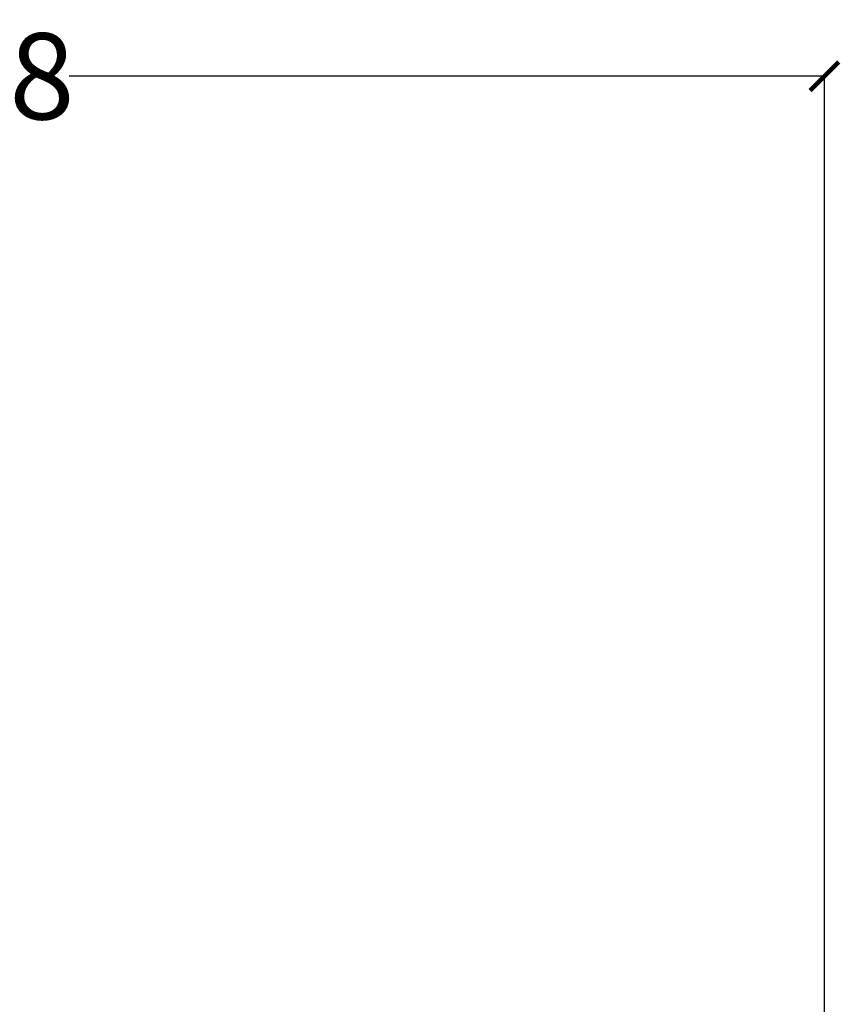
# Model space of a CAD drawing. Units: inches. Extents: x 1704 to 6393, y -157 to 1172.
# Tile 116 of 122: x 2667 to 2724, y 1041 to 1109. Entities that reach past the tile are written whole.
import ezdxf

# ---------------------------------------------------------------- set-up
doc = ezdxf.new("R2010")
doc.units = ezdxf.units.IN
doc.header["$MEASUREMENT"] = 0
doc.layers.add('A-ANNO-DIMS', color=7, linetype='Continuous', lineweight=13)
doc.styles.get("Standard").update_dxf_attribs({"font": 'arial.ttf'})
doc.dimstyles.get("Standard").update_dxf_attribs({"dimtxt": 6, "dimasz": 2, "dimexe": 0.18, "dimexo": 0.0625, "dimgap": 0.09, "dimtad": 0, "dimtih": 1, "dimtoh": 1, "dimdec": 1, "dimzin": 0, "dimdsep": 46, "dimlunit": 3, "dimtxsty": 'Standard', "dimblk": 'ARCHTICK', "dimcen": 0.09, "dimadec": 0, "dimazin": 0, "dimtfac": 1, "dimtdec": 1, "dimtofl": 0, "dimtmove": 0, "dimatfit": 3, "dimfxl": 1, "dimtolj": 1, "dimtzin": 0, "dimarcsym": 0})

# ---------------------------------------------------------------- blocks, each defined once
blk = doc.blocks.new('_ArchTick')
at = {"color": 0, "linetype": 'ByBlock', "const_width": 0.15}
blk.add_lwpolyline([(-0.5, -0.5), (0.5, 0.5)], dxfattribs=at)
blk = doc.blocks.new('*D95')
at = {"layer": 'A-ANNO-DIMS', "color": 0, "lineweight": -2, "transparency": 16777216}
for p, q in [((2605.349, 895.275), (2605.349, 1105.287)), ((2723.349, 895.275), (2723.349, 1105.287)), ((2605.349, 1105.107), (2657.907, 1105.107)), ((2723.349, 1105.107), (2670.791, 1105.107))]:
    blk.add_line(p, q, dxfattribs=at)
at = {"layer": 'Defpoints', "color": 0, "lineweight": -3, "transparency": 16777216}
for p in [(2723.349, 1105.107), (2605.349, 895.213), (2723.349, 895.213)]:
    blk.add_point(p, dxfattribs=at)
at = {"layer": 'A-ANNO-DIMS', "color": 0, "lineweight": -2, "transparency": 16777216, "xscale": 2, "yscale": 2, "zscale": 2, "rotation": 180}
blk.add_blockref('_ArchTick', (2605.349, 1105.107), dxfattribs=at)
at = {"layer": 'A-ANNO-DIMS', "color": 0, "lineweight": -2, "transparency": 16777216, "xscale": 2, "yscale": 2, "zscale": 2}
blk.add_blockref('_ArchTick', (2723.349, 1105.107), dxfattribs=at)
at = {"layer": 'A-ANNO-DIMS', "color": 0, "transparency": 16777216, "insert": (2664.349, 1105.107), "char_height": 6, "attachment_point": 5}
blk.add_mtext('\\A1;118', dxfattribs=at)

msp = doc.modelspace()

# ---------------------------------------------------------------- dimensions: what is measured, and where the dimension line sits
at = {"layer": 'A-ANNO-DIMS'}
dim = msp.add_linear_dim(base=(2723.349, 1105.107), p1=(2605.349, 895.213), p2=(2723.349, 895.213), dimstyle='Standard', override={"dimdec": 0, "dimlfac": 1, "dimrnd": 0, "dimzin": 0, "dimdsep": 46, "dimlunit": 2}, dxfattribs=at)
dim.commit()
dim.dimension.update_dxf_attribs({"geometry": '*D95', "text_midpoint": (2664.349, 1105.107)})

doc.saveas('drawing.dxf')
